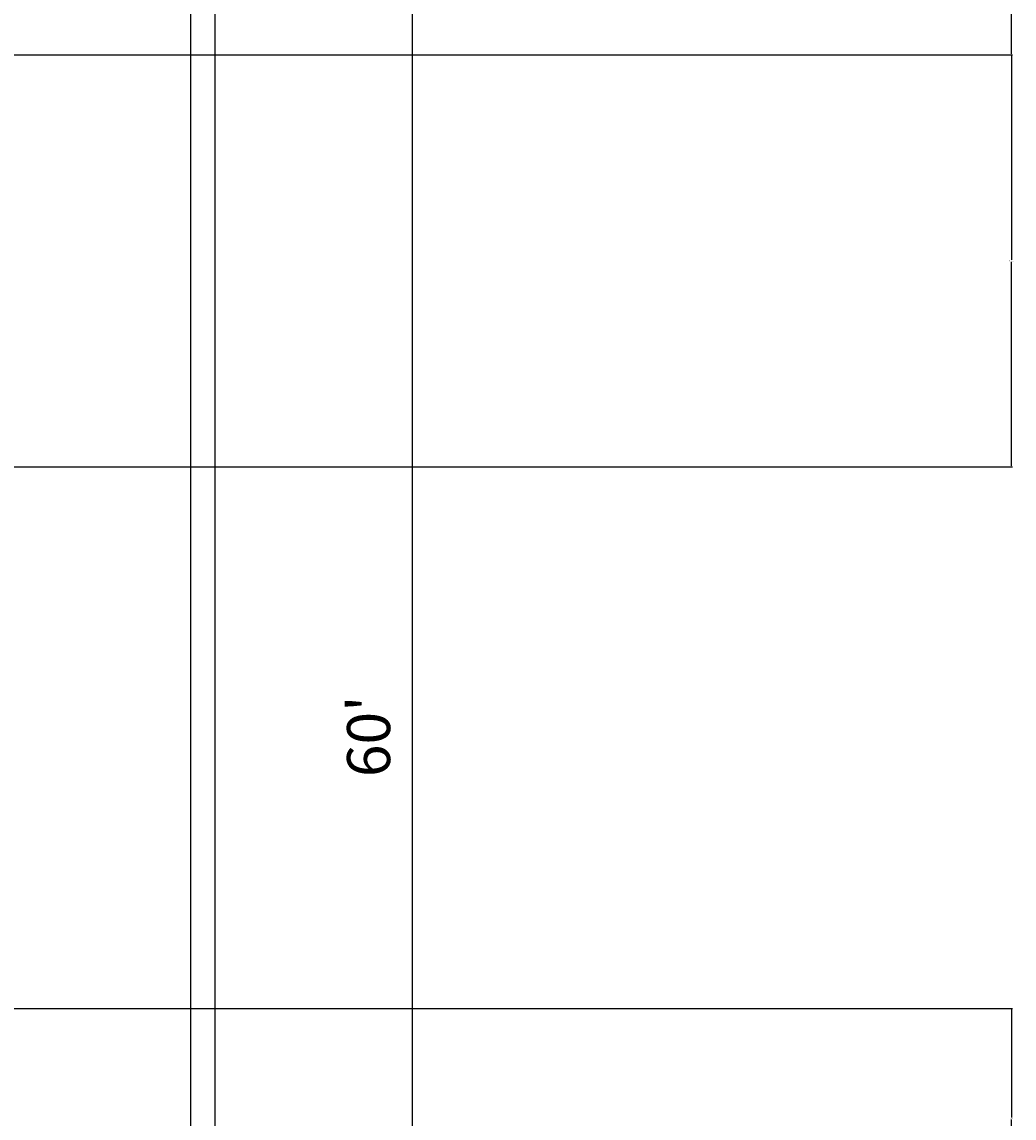
# Model space of a CAD drawing. Units: inches. Extents: x 502 to 1235, y -850 to 110.
# Tile 8 of 9: x 1051 to 1235, y -415 to -212. Entities that reach past the tile are written whole.
import ezdxf

# ---------------------------------------------------------------- set-up
doc = ezdxf.new("R2010")
doc.units = ezdxf.units.IN
doc.header["$MEASUREMENT"] = 0
doc.layers.add('A-ANNO-DIMS', color=2, linetype='Continuous', lineweight=18)
doc.layers.add('C-PROP', color=1, linetype='Continuous', lineweight=25)
doc.styles.get("Standard").update_dxf_attribs({"font": 'arial.ttf'})
doc.dimstyles.get("Standard").update_dxf_attribs({"dimtxt": 0.18, "dimasz": 0.18, "dimexe": 0.18, "dimexo": 0.0625, "dimgap": 0.09, "dimtad": 0, "dimtih": 1, "dimtoh": 1, "dimdec": 1, "dimzin": 0, "dimdsep": 46, "dimlunit": 4, "dimtxsty": 'Standard', "dimcen": 0.09, "dimadec": 0, "dimazin": 0, "dimtfac": 1, "dimtdec": 1, "dimtofl": 0, "dimtmove": 0, "dimatfit": 3, "dimfxl": 1, "dimtolj": 1, "dimtzin": 0, "dimarcsym": 0})

# ---------------------------------------------------------------- blocks, each defined once
blk = doc.blocks.new('_ArchTick')
at = {"color": 0, "linetype": 'ByBlock', "const_width": 0.15}
blk.add_lwpolyline([(-0.5, -0.5), (0.5, 0.5)], dxfattribs=at)
blk = doc.blocks.new('*D6')
at = {"layer": 'A-ANNO-DIMS', "color": 0, "lineweight": -2, "transparency": 16777216}
for p, q in [((1122.49, 15.65), (1123.67, 15.65)), ((1123.49, 15.65), (1123.49, -704.35)), ((1122.49, -704.35), (1123.67, -704.35))]:
    blk.add_line(p, q, dxfattribs=at)
at = {"layer": 'Defpoints', "color": 0, "transparency": 16777216}
for p in [(1086.89, 15.65), (1086.89, -704.35), (1123.49, -704.35)]:
    blk.add_point(p, dxfattribs=at)
at = {"layer": 'A-ANNO-DIMS', "color": 0, "lineweight": -2, "transparency": 16777216, "xscale": 5, "yscale": 5, "zscale": 5}
for p, rotation in [((1123.49, 15.65), 90), ((1123.49, -704.35), 270)]:
    blk.add_blockref('_ArchTick', p, dxfattribs=dict(at, rotation=rotation))
at = {"layer": 'A-ANNO-DIMS', "color": 0, "transparency": 16777216, "insert": (1115.41, -344.35), "char_height": 8, "attachment_point": 5, "rotation": 90}
blk.add_mtext("\\A1;60'", dxfattribs=at)
blk = doc.blocks.new('*D28')
at = {"layer": 'A-ANNO-DIMS', "color": 0, "lineweight": -2, "transparency": 16777216}
for p, q in [((770.85, -217.85), (1235.01, -217.85)), ((1234.83, -218.03), (1234.83, -255.91)), ((1234.83, -294.17), (1234.83, -256.28)), ((770.85, -294.35), (1235.01, -294.35))]:
    blk.add_line(p, q, dxfattribs=at)
at = {"layer": 'A-ANNO-DIMS', "color": 0, "transparency": 16777216}
for points in [[(1234.8, -218.03), (1234.86, -218.03), (1234.83, -217.85)], [(1234.8, -294.17), (1234.86, -294.17), (1234.83, -294.35)]]:
    blk.add_solid(points, dxfattribs=at)
at = {"layer": 'Defpoints', "color": 0, "transparency": 16777216}
for p in [(770.79, -217.85), (770.79, -294.35), (1234.83, -294.35)]:
    blk.add_point(p, dxfattribs=at)
at = {"layer": 'A-ANNO-DIMS', "color": 0, "transparency": 16777216, "insert": (1234.83, -256.1), "char_height": 0.18, "attachment_point": 5}
blk.add_mtext('\\A1;6\'-4 1/2"', dxfattribs=at)
blk = doc.blocks.new('*D29')
at = {"layer": 'A-ANNO-DIMS', "color": 0, "lineweight": -2, "transparency": 16777216}
for p, q in [((644.45, -193.85), (1235.01, -193.85)), ((1234.83, -194.03), (1234.83, -205.66)), ((1234.83, -217.67), (1234.83, -206.03)), ((644.45, -217.85), (1235.01, -217.85))]:
    blk.add_line(p, q, dxfattribs=at)
at = {"layer": 'A-ANNO-DIMS', "color": 0, "transparency": 16777216}
for points in [[(1234.8, -194.03), (1234.86, -194.03), (1234.83, -193.85)], [(1234.8, -217.67), (1234.86, -217.67), (1234.83, -217.85)]]:
    blk.add_solid(points, dxfattribs=at)
at = {"layer": 'Defpoints', "color": 0, "transparency": 16777216}
for p in [(644.39, -193.85), (644.39, -217.85), (1234.83, -217.85)]:
    blk.add_point(p, dxfattribs=at)
at = {"layer": 'A-ANNO-DIMS', "color": 0, "transparency": 16777216, "insert": (1234.83, -205.85), "char_height": 0.18, "attachment_point": 5}
blk.add_mtext('\\A1;2\'-0"', dxfattribs=at)
blk = doc.blocks.new('*D55')
at = {"layer": 'A-ANNO-DIMS', "color": 0, "lineweight": -2, "transparency": 16777216}
for p, q in [((1010.45, -394.85), (1235.01, -394.85)), ((1234.83, -395.03), (1234.83, -415.12)), ((1234.83, -435.56), (1234.83, -415.48)), ((1010.45, -435.74), (1235.01, -435.74))]:
    blk.add_line(p, q, dxfattribs=at)
at = {"layer": 'A-ANNO-DIMS', "color": 0, "transparency": 16777216}
for points in [[(1234.8, -395.03), (1234.86, -395.03), (1234.83, -394.85)], [(1234.8, -435.56), (1234.86, -435.56), (1234.83, -435.74)]]:
    blk.add_solid(points, dxfattribs=at)
at = {"layer": 'Defpoints', "color": 0, "transparency": 16777216}
for p in [(1010.39, -394.85), (1234.83, -394.85), (1010.39, -435.74)]:
    blk.add_point(p, dxfattribs=at)
at = {"layer": 'A-ANNO-DIMS', "color": 0, "transparency": 16777216, "insert": (1234.83, -415.3), "char_height": 0.18, "attachment_point": 5}
blk.add_mtext('\\A1;3\'-5"', dxfattribs=at)

msp = doc.modelspace()

# ---------------------------------------------------------------- linework, layer by layer
at = {"layer": 'C-PROP'}
for p, q in [((1086.89, -704.35), (1086.89, 15.65)), ((1082.39, -699.85), (1082.39, 11.15))]:
    msp.add_line(p, q, dxfattribs=at)

# ---------------------------------------------------------------- dimensions: what is measured, and where the dimension line sits
at = {"layer": 'A-ANNO-DIMS'}
for base, p1, p2, override, picture, middle in [((1123.49, -704.35), (1086.89, 15.65), (1086.89, -704.35), {"dimtxt": 8, "dimasz": 5, "dimgap": 4, "dimtad": 1, "dimtih": 0, "dimblk1": 'ArchTick', "dimblk2": 'ArchTick', "dimsah": 1, "dimclrd": 0, "dimclre": 0, "dimclrt": 0, "dimfxlon": 1}, '*D6', (1115.41, -344.35)), ((1234.83, -217.85), (644.39, -193.85), (644.39, -217.85), {"dimdec": 1, "dimlfac": 1, "dimrnd": 0, "dimzin": 1, "dimdsep": 46, "dimlunit": 4, "dimfrac": 2}, '*D29', (1234.83, -205.85)), ((1234.83, -294.35), (770.79, -217.85), (770.79, -294.35), {"dimdec": 1, "dimlfac": 1, "dimrnd": 0, "dimzin": 1, "dimdsep": 46, "dimlunit": 4, "dimfrac": 2}, '*D28', (1234.83, -256.1)), ((1234.83, -394.85), (1010.39, -435.74), (1010.39, -394.85), {"dimdec": 1, "dimlfac": 1, "dimrnd": 0, "dimzin": 1, "dimdsep": 46, "dimlunit": 4, "dimfrac": 2}, '*D55', (1234.83, -415.3))]:
    dim = msp.add_linear_dim(base=base, p1=p1, p2=p2, angle=90, dimstyle='Standard', override=override, dxfattribs=at)
    dim.commit()
    dim.dimension.update_dxf_attribs({"geometry": picture, "text_midpoint": middle})

doc.saveas('drawing.dxf')
